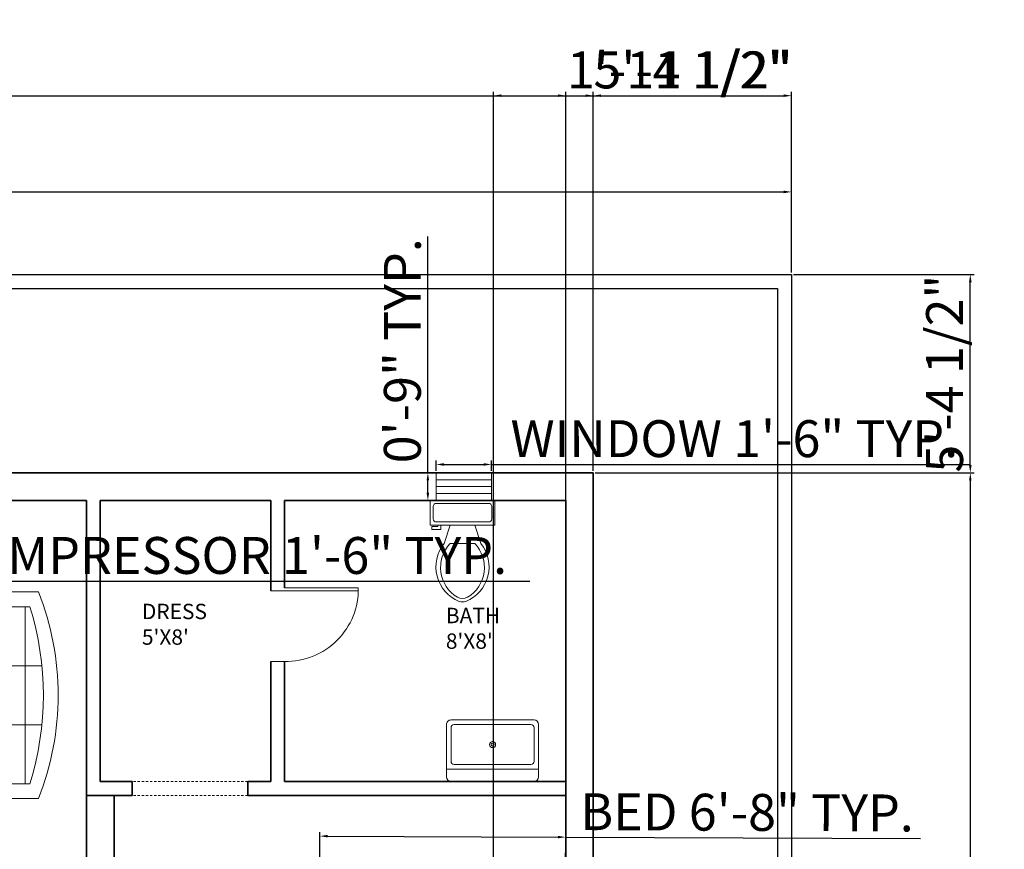
# Model space of a CAD drawing. Units: inches. Extents: x 2562 to 3392, y 1021 to 2243.
# Tile 6 of 6: x 2986 to 3306, y 1973 to 2243. Entities that reach past the tile are written whole.
import ezdxf

# ---------------------------------------------------------------- set-up
doc = ezdxf.new("R2010")
doc.units = ezdxf.units.IN
doc.linetypes.add('JIS_02_0.7', pattern=[1.35, 0.75, -0.6])
for name, color, linetype, lineweight in [('A-ANNO-DIMS', 2, 'Continuous', 18), ('A-AREA-IDEN', 7, 'Continuous', 18), ('A-DOOR', 4, 'Continuous', 18), ('A-FLOR-FIXT', 8, 'Continuous', 18), ('A-FURN', 8, 'Continuous', 18), ('A-GLAZ', 4, 'Continuous', 13), ('A-WALL', 7, 'Continuous', 35), ('A-WALL-HIDN', 7, 'JIS_02_0.7', 18), ('C-PROP', 7, 'Continuous', 30)]:
    doc.layers.add(name, color=color, linetype=linetype, lineweight=lineweight)
doc.styles.get("Standard").update_dxf_attribs({"font": 'arial.ttf'})
doc.dimstyles.new('ISO-25', dxfattribs={"dimtxt": 12, "dimasz": 2.5, "dimexe": 1.25, "dimexo": 0.625, "dimtad": 1, "dimdec": 1, "dimlunit": 3, "dimtxsty": 'Standard', "dimcen": 2.5, "dimadec": 0, "dimazin": 0, "dimtfac": 1, "dimtdec": 1, "dimtmove": 0, "dimatfit": 3, "dimfxl": 1, "dimarcsym": 0})

# ---------------------------------------------------------------- blocks, each defined once
blk = doc.blocks.new('Sofa - Roundback 7 ft.')
for p, q in [((-12.00002, -32.4421), (-12.00003, -6.5971)), ((11.99997, -32.4421), (11.99998, -6.5971)), ((-36.000027, -34), (-36.000027, -11.4696)), ((35.99998, -34), (35.99998, -11.4696)), ((-35.999844, -13.3819), (35.9998, -13.3819)), ((-36.000027, -32.4421), (35.99998, -32.4421))]:
    blk.add_line(p, q)
for points in [[(-36.000027, -34), (-42.000027, -34), (-42.000027, -8)], [(41.99998, -8), (41.99998, -34), (35.99998, -34)]]:
    blk.add_lwpolyline(points)
for centre, radius, start, end in [((0, -114.25), 114.25, 68.43141, 111.5686), ((-0.00001, -127.1968), 121.1968, 72.72033, 107.2797)]:
    blk.add_arc(centre, radius, start, end)
blk = doc.blocks.new('Toilet - top')
for p, q in [((9.5, -6), (9.5, -2)), ((-10, -8.5), (-8, -8.5)), ((-10, -9.5), (-10, -8.5)), ((-7, -9.5), (-10, -9.5)), ((-8, -8.5), (-8, -8)), ((-7, -8), (-7, -9.5)), ((-4, -8), (-6, -14)), ((4, -8), (6, -14)), ((4, -14), (-4, -14))]:
    blk.add_line(p, q)
blk.add_lwpolyline([(10.5, -8), (10.5, 0), (-10.5, 0), (-10.5, -8)], close=True)
for points in [[(-9.5, -2), (-9.5, -6)], [(8.5, -1), (-8.5, -1)], [(-8.5, -7), (8.5, -7)]]:
    blk.add_lwpolyline(points)
for centre, radius, start, end in [((-8.62, -1.88), 0.884, 81.8699, 188.1301), ((8.62, -1.88), 0.884, 351.8699, 98.1301), ((-8.62, -6.12), 0.884, 171.8699, 278.1301), ((8.62, -6.12), 0.884, 261.8699, 8.1301), ((3.52, -21.58), 12.17, 141.4691, 247.9714), ((4.2, -21.82), 11.33, 136.3677, 238.9468), ((-3.52, -21.58), 12.17, 292.0284, 38.5307), ((-4.2, -21.82), 11.33, 301.053, 43.6321), ((0, -27.88), 4, 245.7318, 294.2682), ((0, -29), 4, 254.8605, 285.1395)]:
    blk.add_arc(centre, radius, start, end)
blk = doc.blocks.new('Sink-single - 30 in top')
blk.add_line((-15, -3.999996), (15, -3.999996))
for points in [[(-13.5, 0), (13.5, 0)], [(-15, -18.499996), (-15, -1.5)], [(15, -1.5), (15, -18.499996)], [(-12.5, -5.499996), (12.5, -5.499996)], [(-13.5, -17.499996), (-13.5, -6.499996)], [(13.5, -6.499996), (13.5, -17.499996)], [(12.5, -18.499996), (-12.5, -18.499996)], [(13.5, -19.999996), (-13.5, -19.999996)]]:
    blk.add_lwpolyline(points)
for radius in [1, 0.5]:
    blk.add_circle((0, -11.999996), radius)
for centre, radius, start, end in [((-13.5, -1.5), 1.5, 90, 180), ((13.5, -1.5), 1.5, 0, 90), ((-12.5, -6.499996), 1, 90, 180), ((12.5, -6.499996), 1, 0, 90), ((-13.5, -18.499996), 1.5, 180, 270), ((-12.5, -17.499996), 1, 180, 270), ((12.5, -17.499996), 1, 270, 0), ((13.5, -18.499996), 1.5, 270, 0)]:
    blk.add_arc(centre, radius, start, end)
blk = doc.blocks.new('Window - Wood Frame 36 in. Wide plan')
for p, q in [((0, 6), (0, 0)), ((0, 4.5), (36, 4.5)), ((36, 6), (36, 0)), ((0, 3), (36, 3)), ((0, 1.5), (36, 1.5))]:
    blk.add_line(p, q)
blk = doc.blocks.new('*D21')
at = {"layer": 'A-ANNO-DIMS', "color": 0, "lineweight": -2, "transparency": 16777216}
for p, q in [((2636.76, 2160.76), (2636.76, 2188.27)), ((2639.26, 2187.02), (3234.26, 2187.02)), ((3236.76, 2160.76), (3236.76, 2188.27))]:
    blk.add_line(p, q, dxfattribs=at)
at = {"layer": 'A-ANNO-DIMS', "color": 0, "transparency": 16777216}
for points in [[(2639.26, 2187.43), (2639.26, 2186.6), (2636.76, 2187.02)], [(3234.26, 2187.43), (3234.26, 2186.6), (3236.76, 2187.02)]]:
    blk.add_solid(points, dxfattribs=at)
at = {"layer": 'Defpoints', "color": 0, "transparency": 16777216}
for p in [(3236.76, 2187.02), (2636.76, 2160.13), (3236.76, 2160.13)]:
    blk.add_point(p, dxfattribs=at)
at = {"layer": 'A-ANNO-DIMS', "color": 0, "transparency": 16777216, "insert": (2936.76, 2193.77), "char_height": 12, "attachment_point": 5}
blk.add_mtext("50'", dxfattribs=at)
blk = doc.blocks.new('DOOR-SWING-24IN')
for p, q in [((24.01, 28.5), (23.01, 28.5)), ((23.01, 28.5), (23.01, 0)), ((24.01, 4.5), (24.01, 28.5)), ((0.01, 4.5), (0.01, 0))]:
    blk.add_line(p, q)
blk.add_arc((23.51, 5), 23.51, 88.7811, 181.2189)
blk = doc.blocks.new('*D27')
at = {"layer": 'A-ANNO-DIMS', "color": 0, "lineweight": -2, "transparency": 16777216}
for p, q in [((3121.11, 2096.26), (3121.11, 2099.58)), ((3139.11, 2096.26), (3139.11, 2099.58)), ((3123.61, 2098.33), (3136.61, 2098.33)), ((3139.11, 2098.33), (3294.71, 2098.33))]:
    blk.add_line(p, q, dxfattribs=at)
at = {"layer": 'A-ANNO-DIMS', "color": 0, "transparency": 16777216}
for points in [[(3123.61, 2098.75), (3123.61, 2097.92), (3121.11, 2098.33)], [(3136.61, 2098.75), (3136.61, 2097.92), (3139.11, 2098.33)]]:
    blk.add_solid(points, dxfattribs=at)
at = {"layer": 'Defpoints', "color": 0, "transparency": 16777216}
for p in [(3139.11, 2098.33), (3121.11, 2095.63), (3139.11, 2095.63)]:
    blk.add_point(p, dxfattribs=at)
at = {"layer": 'A-ANNO-DIMS', "color": 0, "transparency": 16777216, "insert": (3218.16, 2105.17), "char_height": 12, "attachment_point": 5}
blk.add_mtext('WINDOW 1\'-6" TYP.', dxfattribs=at)
blk = doc.blocks.new('*D28')
at = {"layer": 'A-ANNO-DIMS', "color": 0, "lineweight": -2, "transparency": 16777216}
for p, q in [((3118.41, 2095.63), (3118.41, 2172.53)), ((3120.48, 2095.63), (3117.16, 2095.63)), ((3118.41, 2089.13), (3118.41, 2093.13)), ((3120.48, 2086.63), (3117.16, 2086.63))]:
    blk.add_line(p, q, dxfattribs=at)
at = {"layer": 'A-ANNO-DIMS', "color": 0, "transparency": 16777216}
for points in [[(3117.99, 2093.13), (3118.82, 2093.13), (3118.41, 2095.63)], [(3117.99, 2089.13), (3118.82, 2089.13), (3118.41, 2086.63)]]:
    blk.add_solid(points, dxfattribs=at)
at = {"layer": 'Defpoints', "color": 0, "transparency": 16777216}
for p in [(3118.41, 2095.63), (3121.11, 2095.63), (3121.11, 2086.63)]:
    blk.add_point(p, dxfattribs=at)
at = {"layer": 'A-ANNO-DIMS', "color": 0, "transparency": 16777216, "insert": (3111.66, 2135.33), "char_height": 12, "attachment_point": 5, "rotation": 90}
blk.add_mtext('0\'-9" TYP.', dxfattribs=at)
blk = doc.blocks.new('*D33')
at = {"layer": 'A-ANNO-DIMS', "color": 0, "lineweight": -2, "transparency": 16777216}
for p, q in [((3083.21, 1966.02), (3083.26, 1978.64)), ((3085.76, 1977.38), (3160.76, 1977.07)), ((3163.21, 1965.69), (3163.26, 1978.31)), ((3163.26, 1977.06), (3278.75, 1976.59))]:
    blk.add_line(p, q, dxfattribs=at)
at = {"layer": 'A-ANNO-DIMS', "color": 0, "transparency": 16777216}
for points in [[(3085.76, 1977.8), (3085.76, 1976.97), (3083.26, 1977.39)], [(3160.76, 1977.49), (3160.76, 1976.66), (3163.26, 1977.06)]]:
    blk.add_solid(points, dxfattribs=at)
at = {"layer": 'Defpoints', "color": 0, "transparency": 16777216}
for p in [(3163.26, 1977.06), (3083.21, 1965.4), (3163.21, 1965.06)]:
    blk.add_point(p, dxfattribs=at)
at = {"layer": 'A-ANNO-DIMS', "color": 0, "transparency": 16777216, "insert": (3222.28, 1983.57), "char_height": 12, "attachment_point": 5, "rotation": 359.7633}
blk.add_mtext('BED 6\'-8" TYP.', dxfattribs=at)
blk = doc.blocks.new('*D41')
at = {"layer": 'A-ANNO-DIMS', "color": 0, "lineweight": -2, "transparency": 16777216}
for p, q in [((2931.06, 2062.4), (2931.06, 2059.08)), ((2949.06, 2062.4), (2949.06, 2059.08)), ((2933.56, 2060.33), (2946.56, 2060.33)), ((2949.06, 2060.33), (3151.56, 2060.33))]:
    blk.add_line(p, q, dxfattribs=at)
at = {"layer": 'A-ANNO-DIMS', "color": 0, "transparency": 16777216}
for points in [[(2933.56, 2060.75), (2933.56, 2059.91), (2931.06, 2060.33)], [(2946.56, 2060.75), (2946.56, 2059.91), (2949.06, 2060.33)]]:
    blk.add_solid(points, dxfattribs=at)
at = {"layer": 'Defpoints', "color": 0, "transparency": 16777216}
for p in [(2931.06, 2063.03), (2949.06, 2063.03), (2949.06, 2060.33)]:
    blk.add_point(p, dxfattribs=at)
at = {"layer": 'A-ANNO-DIMS', "color": 0, "transparency": 16777216, "insert": (3051.56, 2067.16), "char_height": 12, "attachment_point": 5}
blk.add_mtext('COMPRESSOR 1\'-6" TYP.', dxfattribs=at)
blk = doc.blocks.new('*D69')
at = {"layer": 'A-ANNO-DIMS', "color": 0, "lineweight": -2, "transparency": 16777216}
for p, q in [((2701.26, 2096.26), (2701.26, 2219.58)), ((2703.76, 2218.33), (3169.76, 2218.33)), ((3172.26, 2096.26), (3172.26, 2219.58))]:
    blk.add_line(p, q, dxfattribs=at)
at = {"layer": 'A-ANNO-DIMS', "color": 0, "transparency": 16777216}
for points in [[(2703.76, 2218.75), (2703.76, 2217.92), (2701.26, 2218.33)], [(3169.76, 2218.75), (3169.76, 2217.92), (3172.26, 2218.33)]]:
    blk.add_solid(points, dxfattribs=at)
at = {"layer": 'Defpoints', "color": 0, "transparency": 16777216}
for p in [(3172.26, 2218.33), (2701.26, 2095.63), (3172.26, 2095.63)]:
    blk.add_point(p, dxfattribs=at)
at = {"layer": 'A-ANNO-DIMS', "color": 0, "transparency": 16777216, "insert": (2936.76, 2225.09), "char_height": 12, "attachment_point": 5}
blk.add_mtext('39\'-3"', dxfattribs=at)
blk = doc.blocks.new('*D70')
at = {"layer": 'A-ANNO-DIMS', "color": 0, "lineweight": -2, "transparency": 16777216}
for p, q in [((3172.89, 2095.63), (3296.21, 2095.63)), ((3294.96, 2093.13), (3294.96, 1351.49)), ((3114.84, 1348.99), (3296.21, 1348.99))]:
    blk.add_line(p, q, dxfattribs=at)
at = {"layer": 'A-ANNO-DIMS', "color": 0, "transparency": 16777216}
for points in [[(3294.55, 2093.13), (3295.38, 2093.13), (3294.96, 2095.63)], [(3294.55, 1351.49), (3295.38, 1351.49), (3294.96, 1348.99)]]:
    blk.add_solid(points, dxfattribs=at)
at = {"layer": 'Defpoints', "color": 0, "transparency": 16777216}
for p in [(3172.26, 2095.63), (3114.22, 1348.99), (3294.96, 1348.99)]:
    blk.add_point(p, dxfattribs=at)
at = {"layer": 'A-ANNO-DIMS', "color": 0, "transparency": 16777216, "insert": (3288.13, 1722.31), "char_height": 12, "attachment_point": 5, "rotation": 90}
blk.add_mtext('62\'-2 1/2"', dxfattribs=at)
blk = doc.blocks.new('*D71')
at = {"layer": 'A-ANNO-DIMS', "color": 0, "lineweight": -2, "transparency": 16777216}
for p, q in [((3172.26, 2096.26), (3172.26, 2219.58)), ((3174.76, 2218.33), (3234.26, 2218.33)), ((3236.76, 2160.76), (3236.76, 2219.58))]:
    blk.add_line(p, q, dxfattribs=at)
at = {"layer": 'A-ANNO-DIMS', "color": 0, "transparency": 16777216}
for points in [[(3174.76, 2218.75), (3174.76, 2217.92), (3172.26, 2218.33)], [(3234.26, 2218.75), (3234.26, 2217.92), (3236.76, 2218.33)]]:
    blk.add_solid(points, dxfattribs=at)
at = {"layer": 'Defpoints', "color": 0, "transparency": 16777216}
for p in [(3236.76, 2218.33), (3236.76, 2160.13), (3172.26, 2095.63)]:
    blk.add_point(p, dxfattribs=at)
at = {"layer": 'A-ANNO-DIMS', "color": 0, "transparency": 16777216, "insert": (3204.51, 2225.16), "char_height": 12, "attachment_point": 5}
blk.add_mtext('5\'-4 1/2"', dxfattribs=at)
blk = doc.blocks.new('*D72')
at = {"layer": 'A-ANNO-DIMS', "color": 0, "lineweight": -2, "transparency": 16777216}
for p, q in [((3237.39, 2160.13), (3296.21, 2160.13)), ((3294.96, 2098.13), (3294.96, 2157.63)), ((3172.89, 2095.63), (3296.21, 2095.63))]:
    blk.add_line(p, q, dxfattribs=at)
at = {"layer": 'A-ANNO-DIMS', "color": 0, "transparency": 16777216}
for points in [[(3294.55, 2157.63), (3295.38, 2157.63), (3294.96, 2160.13)], [(3294.55, 2098.13), (3295.38, 2098.13), (3294.96, 2095.63)]]:
    blk.add_solid(points, dxfattribs=at)
at = {"layer": 'Defpoints', "color": 0, "transparency": 16777216}
for p in [(3236.76, 2160.13), (3294.96, 2160.13), (3172.26, 2095.63)]:
    blk.add_point(p, dxfattribs=at)
at = {"layer": 'A-ANNO-DIMS', "color": 0, "transparency": 16777216, "insert": (3288.13, 2127.88), "char_height": 12, "attachment_point": 5, "rotation": 90}
blk.add_mtext('5\'-4 1/2"', dxfattribs=at)
blk = doc.blocks.new('*D77')
at = {"layer": 'A-ANNO-DIMS', "color": 0, "lineweight": -2, "transparency": 16777216}
for p, q in [((3139.79, 1809.76), (3139.79, 2219.58)), ((3142.29, 2218.33), (3160.76, 2218.33)), ((3163.26, 1809.76), (3163.26, 2219.58)), ((3163.26, 2218.33), (3235.07, 2218.33))]:
    blk.add_line(p, q, dxfattribs=at)
at = {"layer": 'A-ANNO-DIMS', "color": 0, "transparency": 16777216}
for points in [[(3142.29, 2218.75), (3142.29, 2217.92), (3139.79, 2218.33)], [(3160.76, 2218.75), (3160.76, 2217.92), (3163.26, 2218.33)]]:
    blk.add_solid(points, dxfattribs=at)
at = {"layer": 'Defpoints', "color": 0, "transparency": 16777216}
for p in [(3163.26, 2218.33), (3139.79, 1809.13), (3163.26, 1809.13)]:
    blk.add_point(p, dxfattribs=at)
at = {"layer": 'A-ANNO-DIMS', "color": 0, "transparency": 16777216, "insert": (3200.41, 2225.16), "char_height": 12, "attachment_point": 5}
blk.add_mtext('1\'-11 1/2"', dxfattribs=at)

msp = doc.modelspace()

# ---------------------------------------------------------------- linework, layer by layer
at = {"layer": 'A-WALL'}
for p, q in [((2701.26, 2095.63), (3172.26, 2095.63)), ((3172.26, 2095.63), (3172.26, 1360.63)), ((2818.26, 2086.63), (3007.26, 2086.63)), ((3007.26, 2086.63), (3007.26, 1995.13)), ((3007.26, 2086.63), (3007.26, 1878.13)), ((3011.76, 2086.63), (3011.76, 1995.13)), ((3011.76, 2086.63), (3067.26, 2086.63)), ((3067.26, 2086.63), (3067.26, 2057.23)), ((3071.76, 2086.63), (3071.76, 2058.23)), ((3071.76, 2086.63), (3163.26, 2086.63)), ((3163.26, 2086.63), (3163.26, 1365.13)), ((3007.26, 2034.23), (3007.26, 1990.63)), ((3067.26, 2034.23), (3067.26, 1995.13)), ((3071.76, 2034.23), (3071.76, 1995.13)), ((3011.76, 1995.13), (3022.15, 1995.13)), ((3022.15, 1995.13), (3022.15, 1990.63)), ((3059.77, 1995.13), (3059.77, 1990.63)), ((3059.77, 1995.13), (3067.26, 1995.13)), ((3071.76, 1995.13), (3163.26, 1995.13)), ((3007.26, 1990.63), (3022.15, 1990.63)), ((3016.26, 1990.63), (3016.26, 1839.74)), ((3059.77, 1990.63), (3163.26, 1990.63))]:
    msp.add_line(p, q, dxfattribs=at)
at = {"layer": 'A-WALL-HIDN'}
for p, q in [((3059.77, 1995.13), (3022.15, 1995.13)), ((3059.77, 1990.63), (3022.15, 1990.63))]:
    msp.add_line(p, q, dxfattribs=at)
at = {"layer": 'C-PROP'}
for p, q in [((2636.76, 2160.13), (3236.76, 2160.13)), ((3236.76, 2160.13), (3236.76, 1080.13)), ((2641.26, 2155.63), (3232.26, 2155.63)), ((3232.26, 2155.63), (3232.26, 1084.63))]:
    msp.add_line(p, q, dxfattribs=at)

# ---------------------------------------------------------------- block references
at = {"layer": 'A-DOOR', "extrusion": (0, 0, -1), "zscale": -1, "rotation": 89.99999999999957}
msp.add_blockref('DOOR-SWING-24IN', (-3067.26, 2034.23), dxfattribs=at)
at = {"layer": 'A-FLOR-FIXT'}
msp.add_blockref('Toilet - top', (3129.68, 2086.63), dxfattribs=at)
at = {"layer": 'A-FLOR-FIXT', "rotation": 180}
msp.add_blockref('Sink-single - 30 in top', (3139.46, 1995.19), dxfattribs=at)
at = {"layer": 'A-FURN', "xscale": 0.8, "yscale": 0.8, "rotation": 270}
msp.add_blockref('Sofa - Roundback 7 ft.', (2998.06, 2023.25), dxfattribs=at)
at = {"layer": 'A-GLAZ', "xscale": 0.5, "yscale": 1.5}
msp.add_blockref('Window - Wood Frame 36 in. Wide plan', (3121.11, 2086.63), dxfattribs=at)

# ---------------------------------------------------------------- texts
at = {"layer": 'A-AREA-IDEN', "char_height": 5, "attachment_point": 1}
for s, insert in [("DRESS \\P5'X8'", (3025.34, 2053)), ("BATH \\P8'X8'", (3124.26, 2051.68))]:
    msp.add_mtext(s, dxfattribs=dict(at, insert=insert))

# ---------------------------------------------------------------- dimensions: what is measured, and where the dimension line sits
at = {"layer": 'A-ANNO-DIMS'}
for base, p1, p2, override, picture, middle in [((3163.26, 2218.33), (3139.79, 1809.13), (3163.26, 1809.13), {"dimdec": 1, "dimlfac": 1, "dimrnd": 0, "dimzin": 1, "dimdsep": 46, "dimlunit": 4, "dimfrac": 2}, '*D77', (3200.41, 2225.16)), ((3236.76, 2218.33), (3172.26, 2095.63), (3236.76, 2160.13), {"dimdec": 1, "dimlfac": 1, "dimrnd": 0, "dimzin": 1, "dimdsep": 46, "dimlunit": 4, "dimfrac": 2}, '*D71', (3204.51, 2225.16)), ((3172.26, 2218.33), (2701.26, 2095.63), (3172.26, 2095.63), {"dimdec": 1, "dimlfac": 1, "dimrnd": 0, "dimzin": 1, "dimdsep": 46, "dimlunit": 4, "dimfrac": 2}, '*D69', (2936.76, 2225.09)), ((3236.76, 2187.02), (2636.76, 2160.13), (3236.76, 2160.13), {"dimclrd": 0, "dimclre": 0, "dimclrt": 0}, '*D21', (2936.76, 2193.77))]:
    dim = msp.add_linear_dim(base=base, p1=p1, p2=p2, dimstyle='ISO-25', override=override, dxfattribs=at)
    dim.commit()
    dim.dimension.update_dxf_attribs({"geometry": picture, "text_midpoint": middle})
for base, p1, p2, angle, text, picture, middle in [((3118.41, 2095.63), (3121.11, 2086.63), (3121.11, 2095.63), 90, '<> TYP.', '*D28', (3111.66, 2135.33)), ((3163.26, 1977.06), (3083.21, 1965.4), (3163.21, 1965.06), 359.7633, 'BED <> TYP.', '*D33', (3222.28, 1983.57))]:
    dim = msp.add_linear_dim(base=base, p1=p1, p2=p2, angle=angle, text=text, dimstyle='ISO-25', override={"dimdec": 1, "dimlfac": 1, "dimrnd": 0, "dimzin": 1, "dimdsep": 46, "dimlunit": 4, "dimfrac": 2}, dxfattribs=at)
    dim.commit()
    dim.dimension.update_dxf_attribs({"geometry": picture, "text_midpoint": middle})
for base, p2, picture, middle in [((3294.96, 2160.13), (3236.76, 2160.13), '*D72', (3288.13, 2127.88)), ((3294.96, 1348.99), (3114.22, 1348.99), '*D70', (3288.13, 1722.31))]:
    dim = msp.add_linear_dim(base=base, p1=(3172.26, 2095.63), p2=p2, angle=90, dimstyle='ISO-25', override={"dimdec": 1, "dimlfac": 1, "dimrnd": 0, "dimzin": 1, "dimdsep": 46, "dimlunit": 4, "dimfrac": 2}, dxfattribs=at)
    dim.commit()
    dim.dimension.update_dxf_attribs({"geometry": picture, "text_midpoint": middle})
for base, p1, p2, text, picture, middle in [((3139.11, 2098.33), (3121.11, 2095.63), (3139.11, 2095.63), 'WINDOW <> TYP.', '*D27', (3218.16, 2105.17)), ((2949.06, 2060.33), (2931.06, 2063.03), (2949.06, 2063.03), 'COMPRESSOR <> TYP.', '*D41', (3051.56, 2067.16))]:
    dim = msp.add_linear_dim(base=base, p1=p1, p2=p2, text=text, dimstyle='ISO-25', override={"dimdec": 1, "dimlfac": 1, "dimrnd": 0, "dimzin": 1, "dimdsep": 46, "dimlunit": 4, "dimfrac": 2}, dxfattribs=at)
    dim.commit()
    dim.dimension.update_dxf_attribs({"geometry": picture, "text_midpoint": middle})

doc.saveas('drawing.dxf')
